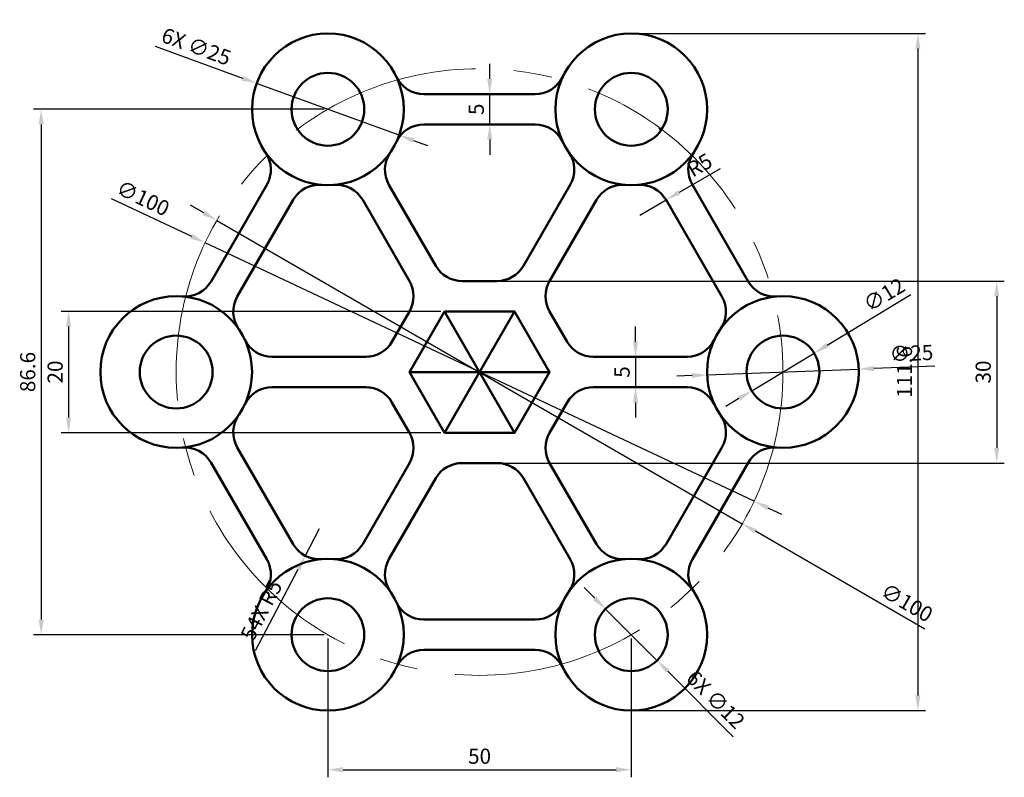
# Model space of a CAD drawing. Units: millimetres. Extents: x -5 to 157, y 7 to 132.
import ezdxf

# ---------------------------------------------------------------- set-up
doc = ezdxf.new("R2010")
doc.units = ezdxf.units.MM
doc.linetypes.add('CENTER', pattern=[50.8, 31.75, -6.35, 6.35, -6.35])
for name, color, linetype, lineweight in [('M-CNTR', 1, 'CENTER', 18), ('M-DIMS', 2, 'Continuous', 25), ('M-OUTL', 7, 'Continuous', 50)]:
    doc.layers.add(name, color=color, linetype=linetype, lineweight=lineweight)
doc.styles.get("Standard").update_dxf_attribs({"font": 'arial.ttf'})
doc.dimstyles.new('ISO-25', dxfattribs={"dimtxt": 2.5, "dimasz": 2.5, "dimexe": 1.25, "dimexo": 0.625, "dimtad": 1, "dimtxsty": 'Standard', "dimcen": 2.5, "dimadec": 0, "dimazin": 0, "dimtfac": 1, "dimtmove": 0, "dimatfit": 3, "dimfxl": 1, "dimarcsym": 0})

# ---------------------------------------------------------------- blocks, each defined once
blk = doc.blocks.new('*D1')
at = {"layer": 'Defpoints', "color": 0, "transparency": 16777216}
for p in [(72.52, 119.61), (80.04, 119.61), (80.04, 114.61)]:
    blk.add_point(p, dxfattribs=at)
at = {"layer": 'M-DIMS', "color": 0, "lineweight": -2, "transparency": 16777216}
for p, q in [((72.52, 122.11), (72.52, 124.61)), ((79.41, 119.61), (71.27, 119.61)), ((72.52, 114.61), (72.52, 119.61)), ((79.41, 114.61), (71.27, 114.61)), ((72.52, 112.11), (72.52, 109.61))]:
    blk.add_line(p, q, dxfattribs=at)
at = {"layer": 'M-DIMS', "color": 0, "transparency": 16777216}
for points in [[(72.11, 122.11), (72.94, 122.11), (72.52, 119.61)], [(72.11, 112.11), (72.94, 112.11), (72.52, 114.61)]]:
    blk.add_solid(points, dxfattribs=at)
at = {"layer": 'M-DIMS', "color": 0, "transparency": 16777216, "insert": (70.63, 117.11), "char_height": 2.5, "attachment_point": 5, "rotation": 90}
blk.add_mtext('5', dxfattribs=at)
blk = doc.blocks.new('*D2')
at = {"layer": 'Defpoints', "color": 0, "transparency": 16777216}
for p in [(89.61, 76.31), (89.61, 71.31), (96.56, 71.31)]:
    blk.add_point(p, dxfattribs=at)
at = {"layer": 'M-DIMS', "color": 0, "lineweight": -2, "transparency": 16777216}
for p, q in [((96.56, 78.81), (96.56, 81.31)), ((90.24, 76.31), (97.81, 76.31)), ((96.56, 76.31), (96.56, 71.31)), ((90.24, 71.31), (97.81, 71.31)), ((96.56, 68.81), (96.56, 66.31))]:
    blk.add_line(p, q, dxfattribs=at)
at = {"layer": 'M-DIMS', "color": 0, "transparency": 16777216}
for points in [[(96.14, 78.81), (96.97, 78.81), (96.56, 76.31)], [(96.14, 68.81), (96.97, 68.81), (96.56, 71.31)]]:
    blk.add_solid(points, dxfattribs=at)
at = {"layer": 'M-DIMS', "color": 0, "transparency": 16777216, "insert": (94.66, 73.81), "char_height": 2.5, "attachment_point": 5, "rotation": 90}
blk.add_mtext('5', dxfattribs=at)
blk = doc.blocks.new('*D3')
at = {"layer": 'Defpoints', "color": 0, "transparency": 16777216}
for p in [(108.36, 73.33), (133.34, 74.29)]:
    blk.add_point(p, dxfattribs=at)
at = {"layer": 'M-DIMS', "color": 0, "lineweight": -2, "transparency": 16777216}
for p, q in [((145.9, 74.78), (135.84, 74.39)), ((105.86, 73.23), (103.36, 73.14)), ((108.36, 73.33), (133.34, 74.29))]:
    blk.add_line(p, q, dxfattribs=at)
at = {"layer": 'M-DIMS', "color": 0, "transparency": 16777216}
for points in [[(135.82, 74.81), (135.85, 73.97), (133.34, 74.29)], [(105.84, 73.65), (105.88, 72.82), (108.36, 73.33)]]:
    blk.add_solid(points, dxfattribs=at)
at = {"layer": 'M-DIMS', "color": 0, "transparency": 16777216, "insert": (142.04, 76.6), "char_height": 2.5, "attachment_point": 5, "rotation": 2.2065}
blk.add_mtext('∅25', dxfattribs=at)
blk = doc.blocks.new('*D4')
at = {"layer": 'Defpoints', "color": 0, "transparency": 16777216}
for p in [(125.99, 76.91), (115.71, 70.71)]:
    blk.add_point(p, dxfattribs=at)
at = {"layer": 'M-DIMS', "color": 0, "lineweight": -2, "transparency": 16777216}
for p, q in [((141.93, 86.53), (128.13, 78.2)), ((115.71, 70.71), (125.99, 76.91)), ((113.57, 69.42), (111.43, 68.13))]:
    blk.add_line(p, q, dxfattribs=at)
at = {"layer": 'M-DIMS', "color": 0, "transparency": 16777216}
for points in [[(127.91, 78.56), (128.34, 77.85), (125.99, 76.91)], [(113.36, 69.78), (113.79, 69.06), (115.71, 70.71)]]:
    blk.add_solid(points, dxfattribs=at)
at = {"layer": 'M-DIMS', "color": 0, "transparency": 16777216, "insert": (137.69, 86.28), "char_height": 2.5, "attachment_point": 5, "rotation": 31.1079}
blk.add_mtext('∅12', dxfattribs=at)
blk = doc.blocks.new('*D5')
at = {"layer": 'Defpoints', "color": 0, "transparency": 16777216}
for p in [(101.59, 102.17), (97.26, 99.67)]:
    blk.add_point(p, dxfattribs=at)
at = {"layer": 'M-DIMS', "color": 0, "lineweight": -2, "transparency": 16777216}
for p, q in [((110.51, 107.32), (103.75, 103.42)), ((97.26, 99.67), (101.59, 102.17))]:
    blk.add_line(p, q, dxfattribs=at)
at = {"layer": 'M-DIMS', "color": 0, "transparency": 16777216}
blk.add_solid([(103.55, 103.78), (103.96, 103.06), (101.59, 102.17)], dxfattribs=at)
at = {"layer": 'M-DIMS', "color": 0, "transparency": 16777216, "insert": (107.27, 107.64), "char_height": 2.5, "attachment_point": 5, "rotation": 30}
blk.add_mtext('R5', dxfattribs=at)
blk = doc.blocks.new('*D6')
at = {"layer": 'Defpoints', "color": 0, "transparency": 16777216}
for p in [(25.61, 95.11), (116.08, 52.51)]:
    blk.add_point(p, dxfattribs=at)
at = {"layer": 'M-DIMS', "color": 0, "lineweight": -2, "transparency": 16777216}
for p, q in [((10.12, 102.41), (23.35, 96.18)), ((116.08, 52.51), (25.61, 95.11)), ((118.34, 51.44), (120.61, 50.38))]:
    blk.add_line(p, q, dxfattribs=at)
at = {"layer": 'M-DIMS', "color": 0, "transparency": 16777216}
for points in [[(23.53, 96.56), (23.17, 95.8), (25.61, 95.11)], [(118.52, 51.82), (118.17, 51.07), (116.08, 52.51)]]:
    blk.add_solid(points, dxfattribs=at)
at = {"layer": 'M-DIMS', "color": 0, "transparency": 16777216, "insert": (15.25, 102.17), "char_height": 2.5, "attachment_point": 5, "rotation": 334.7821}
blk.add_mtext('∅100', dxfattribs=at)
blk = doc.blocks.new('*D7')
at = {"layer": 'Defpoints', "color": 0, "transparency": 16777216}
for p in [(65.07, 83.81), (3.12, 63.81), (65.07, 63.81)]:
    blk.add_point(p, dxfattribs=at)
at = {"layer": 'M-DIMS', "color": 0, "lineweight": -2, "transparency": 16777216}
for p, q in [((64.45, 83.81), (1.87, 83.81)), ((3.12, 81.31), (3.12, 66.31)), ((64.45, 63.81), (1.87, 63.81))]:
    blk.add_line(p, q, dxfattribs=at)
at = {"layer": 'M-DIMS', "color": 0, "transparency": 16777216}
for points in [[(2.7, 81.31), (3.54, 81.31), (3.12, 83.81)], [(2.7, 66.31), (3.54, 66.31), (3.12, 63.81)]]:
    blk.add_solid(points, dxfattribs=at)
at = {"layer": 'M-DIMS', "color": 0, "transparency": 16777216, "insert": (1.22, 73.81), "char_height": 2.5, "attachment_point": 5, "rotation": 90}
blk.add_mtext('20', dxfattribs=at)
blk = doc.blocks.new('*D8')
at = {"layer": 'Defpoints', "color": 0, "transparency": 16777216}
for p in [(73.73, 88.81), (73.73, 58.81), (156.08, 58.81)]:
    blk.add_point(p, dxfattribs=at)
at = {"layer": 'M-DIMS', "color": 0, "lineweight": -2, "transparency": 16777216}
for p, q in [((74.36, 88.81), (157.33, 88.81)), ((156.08, 86.31), (156.08, 61.31)), ((74.36, 58.81), (157.33, 58.81))]:
    blk.add_line(p, q, dxfattribs=at)
at = {"layer": 'M-DIMS', "color": 0, "transparency": 16777216}
for points in [[(155.66, 86.31), (156.5, 86.31), (156.08, 88.81)], [(155.66, 61.31), (156.5, 61.31), (156.08, 58.81)]]:
    blk.add_solid(points, dxfattribs=at)
at = {"layer": 'M-DIMS', "color": 0, "transparency": 16777216, "insert": (154.18, 73.81), "char_height": 2.5, "attachment_point": 5, "rotation": 90}
blk.add_mtext('30', dxfattribs=at)
blk = doc.blocks.new('BOSS-D25-HOLE')
for radius in [12.5, 6]:
    blk.add_circle((120.85, 73.81), radius)
blk = doc.blocks.new('*D10')
at = {"layer": 'Defpoints', "color": 0, "transparency": 16777216}
for p in [(95.85, 129.61), (95.85, 18.01), (143.1, 18.01)]:
    blk.add_point(p, dxfattribs=at)
at = {"layer": 'M-DIMS', "color": 0, "lineweight": -2, "transparency": 16777216}
for p, q in [((96.47, 129.61), (144.35, 129.61)), ((143.1, 127.11), (143.1, 20.51)), ((96.47, 18.01), (144.35, 18.01))]:
    blk.add_line(p, q, dxfattribs=at)
at = {"layer": 'M-DIMS', "color": 0, "transparency": 16777216}
for points in [[(142.68, 127.11), (143.51, 127.11), (143.1, 129.61)], [(142.68, 20.51), (143.51, 20.51), (143.1, 18.01)]]:
    blk.add_solid(points, dxfattribs=at)
at = {"layer": 'M-DIMS', "color": 0, "transparency": 16777216, "insert": (141.2, 73.81), "char_height": 2.5, "attachment_point": 5, "rotation": 90}
blk.add_mtext('111.6', dxfattribs=at)
blk = doc.blocks.new('*D11')
at = {"layer": 'Defpoints', "color": 0, "transparency": 16777216}
for p in [(45.85, 30.51), (95.85, 30.51), (95.85, 8.26)]:
    blk.add_point(p, dxfattribs=at)
at = {"layer": 'M-DIMS', "color": 0, "lineweight": -2, "transparency": 16777216}
for p, q in [((45.85, 29.88), (45.85, 7.01)), ((95.85, 29.88), (95.85, 7.01)), ((48.35, 8.26), (93.35, 8.26))]:
    blk.add_line(p, q, dxfattribs=at)
at = {"layer": 'M-DIMS', "color": 0, "transparency": 16777216}
for points in [[(48.35, 8.68), (48.35, 7.84), (45.85, 8.26)], [(93.35, 8.68), (93.35, 7.84), (95.85, 8.26)]]:
    blk.add_solid(points, dxfattribs=at)
at = {"layer": 'M-DIMS', "color": 0, "transparency": 16777216, "insert": (70.85, 10.16), "char_height": 2.5, "attachment_point": 5}
blk.add_mtext('50', dxfattribs=at)
blk = doc.blocks.new('*D12')
at = {"layer": 'Defpoints', "color": 0, "transparency": 16777216}
for p in [(45.85, 117.11), (-1.4, 30.51), (45.85, 30.51)]:
    blk.add_point(p, dxfattribs=at)
at = {"layer": 'M-DIMS', "color": 0, "lineweight": -2, "transparency": 16777216}
for p, q in [((45.22, 117.11), (-2.65, 117.11)), ((-1.4, 114.61), (-1.4, 33.01)), ((45.22, 30.51), (-2.65, 30.51))]:
    blk.add_line(p, q, dxfattribs=at)
at = {"layer": 'M-DIMS', "color": 0, "transparency": 16777216}
for points in [[(-1.82, 114.61), (-0.99, 114.61), (-1.4, 117.11)], [(-1.82, 33.01), (-0.99, 33.01), (-1.4, 30.51)]]:
    blk.add_solid(points, dxfattribs=at)
at = {"layer": 'M-DIMS', "color": 0, "transparency": 16777216, "insert": (-3.3, 73.81), "char_height": 2.5, "attachment_point": 5, "rotation": 90}
blk.add_mtext('86.6', dxfattribs=at)
blk = doc.blocks.new('*D13')
at = {"layer": 'Defpoints', "color": 0, "transparency": 16777216}
for p in [(34.1, 121.39), (57.59, 112.84)]:
    blk.add_point(p, dxfattribs=at)
at = {"layer": 'M-DIMS', "color": 0, "lineweight": -2, "transparency": 16777216}
for p, q in [((17.36, 127.49), (31.75, 122.24)), ((57.59, 112.84), (34.1, 121.39)), ((59.94, 111.98), (62.29, 111.13))]:
    blk.add_line(p, q, dxfattribs=at)
at = {"layer": 'M-DIMS', "color": 0, "transparency": 16777216}
for points in [[(31.9, 122.64), (31.61, 121.85), (34.1, 121.39)], [(60.09, 112.37), (59.8, 111.59), (57.59, 112.84)]]:
    blk.add_solid(points, dxfattribs=at)
at = {"layer": 'M-DIMS', "color": 0, "transparency": 16777216, "insert": (24.05, 127.15), "char_height": 2.5, "attachment_point": 5, "rotation": 339.9933}
blk.add_mtext('6X ∅25', dxfattribs=at)
blk = doc.blocks.new('*D14')
at = {"layer": 'Defpoints', "color": 0, "transparency": 16777216}
for p in [(91.6, 34.75), (100.09, 26.27)]:
    blk.add_point(p, dxfattribs=at)
at = {"layer": 'M-DIMS', "color": 0, "lineweight": -2, "transparency": 16777216}
for p, q in [((89.84, 36.52), (88.07, 38.29)), ((91.6, 34.75), (100.09, 26.27)), ((112.67, 13.7), (101.86, 24.5))]:
    blk.add_line(p, q, dxfattribs=at)
at = {"layer": 'M-DIMS', "color": 0, "transparency": 16777216}
for points in [[(90.13, 36.81), (89.54, 36.22), (91.6, 34.75)], [(102.15, 24.8), (101.57, 24.21), (100.09, 26.27)]]:
    blk.add_solid(points, dxfattribs=at)
at = {"layer": 'M-DIMS', "color": 0, "transparency": 16777216, "insert": (109.54, 19.61), "char_height": 2.5, "attachment_point": 5, "rotation": 315.0137}
blk.add_mtext('6X ∅12', dxfattribs=at)
blk = doc.blocks.new('*D15')
at = {"layer": 'Defpoints', "color": 0, "transparency": 16777216}
for p in [(27.55, 98.81), (114.15, 48.81)]:
    blk.add_point(p, dxfattribs=at)
at = {"layer": 'M-DIMS', "color": 0, "lineweight": -2, "transparency": 16777216}
for p, q in [((25.38, 100.06), (23.22, 101.31)), ((27.55, 98.81), (114.15, 48.81)), ((144.24, 31.44), (116.31, 47.56))]:
    blk.add_line(p, q, dxfattribs=at)
at = {"layer": 'M-DIMS', "color": 0, "transparency": 16777216}
for points in [[(25.59, 100.42), (25.17, 99.7), (27.55, 98.81)], [(116.52, 47.92), (116.11, 47.2), (114.15, 48.81)]]:
    blk.add_solid(points, dxfattribs=at)
at = {"layer": 'M-DIMS', "color": 0, "transparency": 16777216, "insert": (141.12, 35.52), "char_height": 2.5, "attachment_point": 5, "rotation": 329.9992}
blk.add_mtext('∅100', dxfattribs=at)
blk = doc.blocks.new('*D16')
at = {"layer": 'Defpoints', "color": 0, "transparency": 16777216}
for p in [(44.44, 47.95), (42.11, 43.53)]:
    blk.add_point(p, dxfattribs=at)
at = {"layer": 'M-DIMS', "color": 0, "lineweight": -2, "transparency": 16777216}
for p, q in [((44.44, 47.95), (42.11, 43.53)), ((33.93, 27.93), (40.95, 41.31))]:
    blk.add_line(p, q, dxfattribs=at)
at = {"layer": 'M-DIMS', "color": 0, "transparency": 16777216}
blk.add_solid([(40.58, 41.51), (41.32, 41.12), (42.11, 43.53)], dxfattribs=at)
at = {"layer": 'M-DIMS', "color": 0, "transparency": 16777216, "insert": (35.18, 34.39), "char_height": 2.5, "attachment_point": 5, "rotation": 62.3131}
blk.add_mtext('54X R5', dxfattribs=at)

msp = doc.modelspace()

# ---------------------------------------------------------------- linework, layer by layer
at = {"layer": 'M-CNTR'}
msp.add_circle((70.848, 73.811), 50, dxfattribs=at)
at = {"layer": 'M-OUTL'}
for p, q in [((61.659, 119.613), (80.037, 119.613)), ((93.652, 118.308), (93.683, 118.363)), ((97.982, 115.808), (98.013, 115.863)), ((61.659, 114.613), (80.037, 114.613)), ((100.485, 114.081), (100.74, 113.639)), ((100.485, 114.081), (100.74, 113.639)), ((35.777, 104.669), (26.589, 88.754)), ((105.919, 104.669), (115.107, 88.754)), ((105.919, 104.669), (115.107, 88.754)), ((40.107, 102.169), (30.919, 86.254)), ((101.589, 102.169), (110.777, 86.254)), ((65.074, 63.811), (76.621, 83.811)), ((65.074, 83.811), (76.621, 63.811)), ((65.074, 83.811), (76.621, 63.811)), ((76.621, 83.811), (65.074, 63.811)), ((120.785, 76.311), (120.848, 76.311)), ((59.301, 73.811), (82.395, 73.811)), ((59.301, 73.811), (82.395, 73.811)), ((120.785, 71.311), (120.848, 71.311)), ((40.107, 45.453), (30.919, 61.368)), ((110.777, 61.368), (101.589, 45.453)), ((35.777, 42.953), (26.589, 58.868)), ((115.107, 58.868), (105.919, 42.953)), ((61.659, 33.01), (80.037, 33.01)), ((61.659, 28.01), (80.037, 28.01))]:
    msp.add_line(p, q, dxfattribs=at)
for points in [[(55.919, 104.669), (63.631, 91.311, 0.2679492), (67.961, 88.811)], [(85.777, 104.669), (78.065, 91.311, -0.2679492), (73.735, 88.811)], [(59.301, 83.811, 0.2679492), (59.301, 88.811), (51.589, 102.169)], [(82.395, 83.811, -0.2679492), (82.395, 88.811), (90.107, 102.169)], [(36.659, 76.311), (52.084, 76.311, 0.2679492), (56.414, 78.811)], [(105.037, 76.311), (89.612, 76.311, -0.2679492), (85.282, 78.811)], [(56.414, 68.811, 0.2679492), (52.084, 71.311), (36.659, 71.311)], [(85.282, 68.811, -0.2679492), (89.612, 71.311), (105.037, 71.311)], [(51.589, 45.453), (59.301, 58.811, 0.2679492), (59.301, 63.811)], [(82.395, 63.811, 0.2679492), (82.395, 58.811), (90.107, 45.453)], [(67.961, 58.811, 0.2679492), (63.631, 56.311), (55.919, 42.953)], [(85.777, 42.953), (78.065, 56.311, 0.2679492), (73.735, 58.811)]]:
    msp.add_lwpolyline(points, format="xyb", dxfattribs=at)
for points in [[(73.735, 88.811), (67.961, 88.811)], [(59.301, 83.811), (56.414, 78.811)], [(85.282, 78.811), (82.395, 83.811)], [(56.414, 68.811), (59.301, 63.811)], [(82.395, 63.811), (85.282, 68.811)], [(67.961, 58.811), (73.735, 58.811)]]:
    msp.add_lwpolyline(points, dxfattribs=at)
msp.add_lwpolyline([(65.074, 83.811), (59.301, 73.811), (65.074, 63.811), (76.621, 63.811), (82.395, 73.811), (76.621, 83.811)], close=True, dxfattribs=at)
for centre, start, end in [((61.659, 124.613), 205.37693, 270), ((80.037, 124.613), 270, 334.62307), ((61.659, 109.613), 90, 154.62307), ((80.037, 109.613), 25.37693, 90), ((31.447, 107.169), 330, 34.62307), ((60.249, 107.169), 145.37693, 210), ((81.447, 107.169), 330, 34.62307), ((110.249, 107.169), 145.37693, 210), ((44.437, 99.669), 85.37693, 150), ((47.258, 99.669), 30, 94.62307), ((94.437, 99.669), 85.37693, 150), ((97.258, 99.669), 30, 94.62307), ((22.258, 91.254), 265.37693, 330), ((119.437, 91.254), 210, 274.62307), ((35.249, 83.754), 150, 214.62307), ((106.447, 83.754), 325.37693, 30), ((36.659, 81.311), 205.37693, 270), ((36.659, 81.311), 205.37693, 270), ((105.037, 81.311), 270, 334.62307), ((36.659, 66.311), 90, 154.62307), ((36.659, 66.311), 90, 154.62307), ((105.037, 66.311), 25.37693, 90), ((35.249, 63.868), 145.37693, 210), ((106.447, 63.868), 330, 34.62307), ((22.258, 56.368), 30, 94.62307), ((119.437, 56.368), 85.37693, 150), ((44.437, 47.953), 210, 274.62307), ((47.258, 47.953), 265.37693, 330), ((47.258, 47.953), 265.37693, 330), ((94.437, 47.953), 210, 274.62307), ((94.437, 47.953), 210, 274.62307), ((97.258, 47.953), 265.37693, 330), ((31.447, 40.453), 325.37693, 30), ((60.249, 40.453), 150, 214.62307), ((60.249, 40.453), 150, 214.62307), ((81.447, 40.453), 325.37693, 30), ((81.447, 40.453), 325.37693, 30), ((110.249, 40.453), 150, 214.62307), ((61.659, 38.01), 205.37693, 270), ((80.037, 38.01), 270, 334.62307), ((61.659, 23.01), 90, 154.62307), ((80.037, 23.01), 25.37693, 90)]:
    msp.add_arc(centre, 5, start, end, dxfattribs=at)

# ---------------------------------------------------------------- block references
for p in [(-75, 43.301), (-25, 43.301), (-100, 0), (0, 0), (-75, -43.301), (-25, -43.301)]:
    msp.add_blockref('BOSS-D25-HOLE', p, dxfattribs=at)

# ---------------------------------------------------------------- dimensions: what is measured, and where the dimension line sits
at = {"layer": 'M-DIMS'}
dim = msp.add_diameter_dim_2p(p1=(57.594, 112.836), p2=(34.102, 121.389), text='6X <>', dimstyle='ISO-25', override={"dimdec": 0, "dimlfac": 1, "dimrnd": 0, "dimzin": 0, "dimdsep": 46, "dimlunit": 2}, dxfattribs=at)
dim.commit()
dim.dimension.update_dxf_attribs({"geometry": '*D13', "text_midpoint": (23.38, 125.293), "dimtype": 163})
for base, p1, p2, override, picture, middle in [((143.098, 18.01), (95.848, 129.613), (95.848, 18.01), {"dimdec": 1, "dimlfac": 1, "dimrnd": 0, "dimzin": 0, "dimdsep": 46, "dimlunit": 2}, '*D10', (141.197, 73.811)), ((72.523, 119.613), (80.037, 114.613), (80.037, 119.613), {"dimclrd": 0, "dimclre": 0, "dimclrt": 0}, '*D1', (70.627, 117.113)), ((-1.402, 30.51), (45.848, 117.113), (45.848, 30.51), {"dimdec": 1, "dimlfac": 1, "dimrnd": 0, "dimzin": 0, "dimdsep": 46, "dimlunit": 2}, '*D12', (-3.303, 73.811)), ((156.081, 58.811), (73.735, 88.811), (73.735, 58.811), {"dimclrd": 0, "dimclre": 0, "dimclrt": 0}, '*D8', (154.179, 73.811)), ((3.119, 63.811), (65.074, 83.811), (65.074, 63.811), {"dimclrd": 0, "dimclre": 0, "dimclrt": 0}, '*D7', (1.218, 73.811)), ((96.557, 71.311), (89.612, 76.311), (89.612, 71.311), {"dimclrd": 0, "dimclre": 0, "dimclrt": 0}, '*D2', (94.661, 73.811))]:
    dim = msp.add_linear_dim(base=base, p1=p1, p2=p2, angle=90, dimstyle='ISO-25', override=override, dxfattribs=at)
    dim.commit()
    dim.dimension.update_dxf_attribs({"geometry": picture, "text_midpoint": middle})
dim = msp.add_radius_dim(center=(97.258, 99.669), mpoint=(101.589, 102.169), dimstyle='ISO-25', override={"dimclrd": 0, "dimclre": 0, "dimclrt": 0}, dxfattribs=at)
dim.commit()
dim.dimension.update_dxf_attribs({"geometry": '*D5', "text_midpoint": (107.266, 107.637)})
for p1, p2, override, picture, middle in [((116.083, 52.508), (25.613, 95.114), {"dimclrd": 0, "dimclre": 0, "dimclrt": 0}, '*D6', (14.411, 100.39)), ((27.547, 98.812), (114.149, 48.811), {"dimdec": 0, "dimlfac": 1, "dimrnd": 0, "dimzin": 0, "dimdsep": 46, "dimlunit": 2}, '*D15', (140.129, 33.81)), ((115.711, 70.711), (125.985, 76.911), {"dimclrd": 0, "dimclre": 0, "dimclrt": 0}, '*D4', (138.706, 84.587)), ((108.357, 73.33), (133.339, 74.293), {"dimclrd": 0, "dimclre": 0, "dimclrt": 0}, '*D3', (142.117, 74.631))]:
    dim = msp.add_diameter_dim_2p(p1=p1, p2=p2, dimstyle='ISO-25', override=override, dxfattribs=at)
    dim.commit()
    dim.dimension.update_dxf_attribs({"geometry": picture, "text_midpoint": middle, "dimtype": 163})
dim = msp.add_radius_dim(center=(44.437, 47.953), mpoint=(42.114, 43.526), text='54X <>', dimstyle='ISO-25', override={"dimdec": 0, "dimlfac": 1, "dimrnd": 0, "dimzin": 0, "dimdsep": 46, "dimlunit": 2}, dxfattribs=at)
dim.commit()
dim.dimension.update_dxf_attribs({"geometry": '*D16', "text_midpoint": (35.181, 34.394)})
dim = msp.add_diameter_dim_2p(p1=(91.604, 34.752), p2=(100.092, 26.268), text='6X <>', dimstyle='ISO-25', override={"dimdec": 0, "dimlfac": 1, "dimrnd": 0, "dimzin": 0, "dimdsep": 46, "dimlunit": 2}, dxfattribs=at)
dim.commit()
dim.dimension.update_dxf_attribs({"geometry": '*D14', "text_midpoint": (108.147, 18.217)})
dim = msp.add_linear_dim(base=(95.848, 8.26), p1=(45.848, 30.51), p2=(95.848, 30.51), dimstyle='ISO-25', override={"dimdec": 0, "dimlfac": 1, "dimrnd": 0, "dimzin": 0, "dimdsep": 46, "dimlunit": 2}, dxfattribs=at)
dim.commit()
dim.dimension.update_dxf_attribs({"geometry": '*D11', "text_midpoint": (70.848, 10.161)})

doc.saveas('drawing.dxf')
